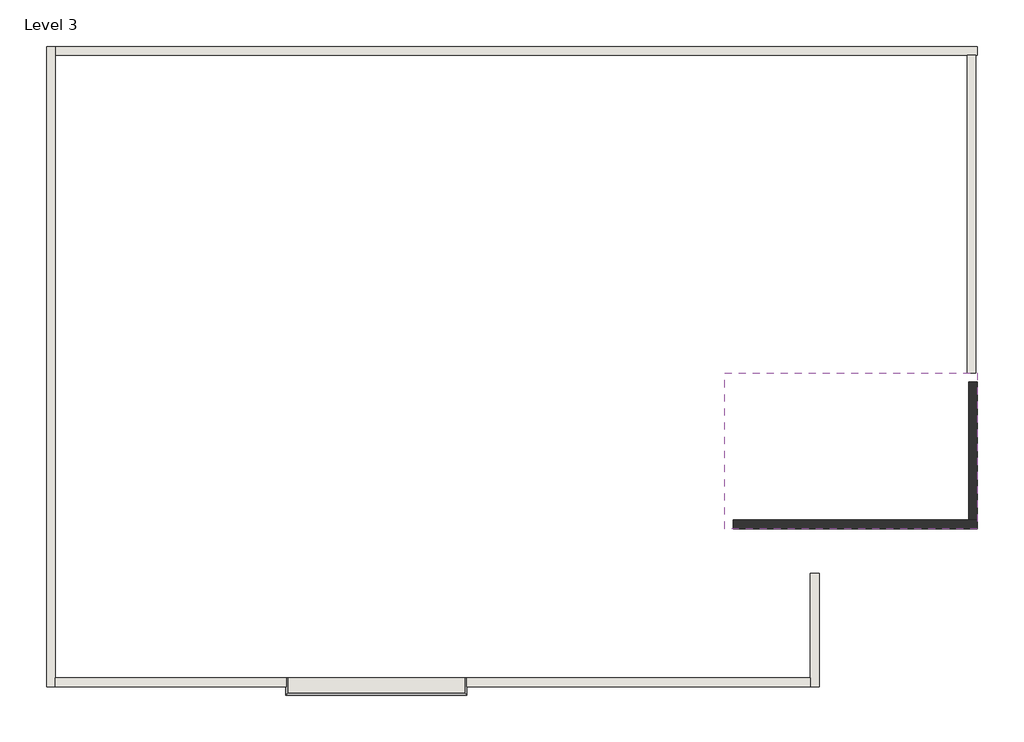
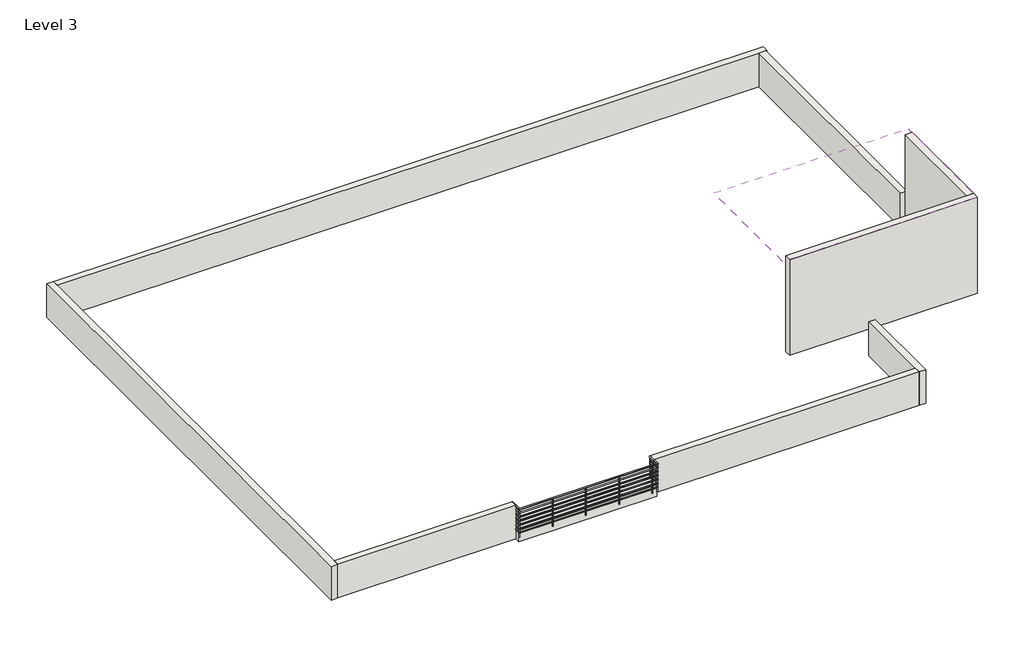
# One storey: 10 walls, 1 covering, 1 railing.
"""IFC4 building model written with IfcOpenShell, lengths in millimetres."""

from ifc_helpers import new_model, si_unit, point, frame, frame_2d, origin, place, context, project, spatial, polyline, circle_curve, ellipse_curve, trimmed, segment, composite_curve, outline, extrude, faceted_brep, transform, mapped, element, save
from ifc_brep_helpers import plane_surface, cylinder_surface, advanced_brep
from components import walls_5_walls_5_63f74a62, walls_6_walls_6_8e6cdcdd

model = new_model("IFC4")

# Units and contexts
model_context = context("Model", 3, world=origin())
ifc_project = project(units=[si_unit("LENGTHUNIT", "METRE", prefix="MILLI")], contexts=[model_context])

# Site, building, storey
site = spatial("IfcSite", under=ifc_project)
building = spatial("IfcBuilding", under=site)
storey = spatial("IfcBuildingStorey", under=building, Name="Level 3", Elevation=3048.0)

# Covering
placement = place(None, origin())
element("IfcCovering", 1, ObjectType="600 x 1200mm grid", at=placement, inside=storey, context=model_context, shape_type="SweptSolid", body=[
    extrude(outline(polyline([(13293.8008502, 3643.3156744), (13293.8008502, 38.1156744), (7439.6639497, 38.1156744), (7439.6639497, 3643.3156744), (13293.8008502, 3643.3156744)])), frame((0.0, 0.0, 6096.0), z_axis=(0.0, 0.0, 1.0), x_axis=(1.0, 0.0, 0.0)), (0.0, 0.0, 1.0), 52.0),
])

# Railing
element("IfcRailing", 2, ObjectType="900mm Pipe", at=placement, inside=storey, context=model_context, shape_type="SolidModel", body=[
    advanced_brep(
    [(-2720.3062226, -3420.8536983, 4095.5083956), (-2680.3062226, -3420.8536983, 4095.5083956), (-2720.3062226, -3815.4929435, 4095.5083956), (-2680.3062226, -3775.4929435, 4095.5083956), (1468.5864069, -3815.4929435, 4095.5083956), (1428.5864069, -3775.4929435, 4095.5083956), (1468.5864069, -3420.8536983, 4095.5083956), (1428.5864069, -3420.8536983, 4095.5083956)],
    [
        (0, 1, circle_curve(frame((-2700.3062226, -3420.8536983, 4095.5083956), z_axis=(0.0, 1.0, 0.0), x_axis=(1.0, 0.0, 0.0)), 20.0)),
        (1, 0, circle_curve(frame((-2700.3062226, -3420.8536983, 4095.5083956), z_axis=(0.0, 1.0, 0.0), x_axis=(1.0, 0.0, 0.0)), 20.0)),
        (0, 2),
        (2, 3, ellipse_curve(frame((-2700.3062226, -3795.4929435, 4095.5083956), z_axis=(-0.7071067811865459, 0.7071067811865491, 0.0), x_axis=(0.7071067811865491, 0.7071067811865458, 0.0)), 28.2842712, 20.0)),
        (3, 1),
        (3, 2, ellipse_curve(frame((-2700.3062226, -3795.4929435, 4095.5083956), z_axis=(-0.7071067811865459, 0.7071067811865491, 0.0), x_axis=(0.7071067811865491, 0.7071067811865458, 0.0)), 28.2842712, 20.0)),
        (2, 4),
        (4, 5, ellipse_curve(frame((1448.5864069, -3795.4929435, 4095.5083956), z_axis=(-0.707106781186549, -0.7071067811865458, 0.0), x_axis=(-0.7071067811865461, 0.7071067811865489, 0.0)), 28.2842712, 20.0)),
        (5, 3),
        (5, 4, ellipse_curve(frame((1448.5864069, -3795.4929435, 4095.5083956), z_axis=(-0.707106781186549, -0.7071067811865458, 0.0), x_axis=(-0.7071067811865461, 0.7071067811865489, 0.0)), 28.2842712, 20.0)),
        (6, 7, circle_curve(frame((1448.5864069, -3420.8536983, 4095.5083956), z_axis=(0.0, 1.0, 0.0), x_axis=(-1.0, 0.0, 0.0)), 20.0)),
        (7, 6, circle_curve(frame((1448.5864069, -3420.8536983, 4095.5083956), z_axis=(0.0, 1.0, 0.0), x_axis=(-1.0, 0.0, 0.0)), 20.0)),
        (4, 6),
        (7, 5),
    ],
    [
        plane_surface(frame((-2700.3062226, -3420.8536983, 4115.5083956), z_axis=(0.0, 1.0, 0.0), x_axis=(0.0, 0.0, -1.0))),
        cylinder_surface(frame((-2700.3062226, -3420.8536983, 4095.5083956), z_axis=(0.0, 1.0, 0.0), x_axis=(1.0, 0.0, 0.0)), 20.0),
        cylinder_surface(frame((-2700.3062226, -3795.4929435, 4095.5083956), z_axis=(-1.0, 0.0, 0.0), x_axis=(0.0, 1.0, 0.0)), 20.0),
        plane_surface(frame((1448.5864069, -3420.8536983, 4115.5083956), z_axis=(0.0, 1.0, 0.0), x_axis=(0.0, 0.0, 1.0))),
        cylinder_surface(frame((1448.5864069, -3795.4929435, 4095.5083956), z_axis=(0.0, -1.0, 0.0), x_axis=(-1.0, 0.0, 0.0)), 20.0),
    ],
    [
        (0, [[1, 2]]),
        (1, [[-1, 3, 4, 5]]),
        (1, [[-2, -5, 6, -3]]),
        (2, [[-4, 7, 8, 9]]),
        (2, [[-6, -9, 10, -7]]),
        (3, [[11, 12]]),
        (4, [[-8, 13, -12, 14]]),
        (4, [[-10, -14, -11, -13]]),
    ],
),
    advanced_brep(
    [(-2685.3062226, -3420.8536983, 3975.5083956), (-2715.3062226, -3420.8536983, 3975.5083956), (-2685.3062226, -3780.4929435, 3975.5083956), (-2715.3062226, -3810.4929435, 3975.5083956), (1433.5864069, -3780.4929435, 3975.5083956), (1463.5864069, -3810.4929435, 3975.5083956), (1433.5864069, -3420.8536983, 3975.5083956), (1463.5864069, -3420.8536983, 3975.5083956)],
    [
        (0, 1, circle_curve(frame((-2700.3062226, -3420.8536983, 3975.5083956), z_axis=(0.0, 1.0, 0.0), x_axis=(-1.0, 0.0, 0.0)), 15.0)),
        (1, 0, circle_curve(frame((-2700.3062226, -3420.8536983, 3975.5083956), z_axis=(0.0, 1.0, 0.0), x_axis=(-1.0, 0.0, 0.0)), 15.0)),
        (0, 2),
        (2, 3, ellipse_curve(frame((-2700.3062226, -3795.4929435, 3975.5083956), z_axis=(-0.7071067811865459, 0.7071067811865491, 0.0), x_axis=(0.7071067811865491, 0.7071067811865458, 0.0)), 21.2132034, 15.0)),
        (3, 1),
        (3, 2, ellipse_curve(frame((-2700.3062226, -3795.4929435, 3975.5083956), z_axis=(-0.7071067811865459, 0.7071067811865491, 0.0), x_axis=(0.7071067811865491, 0.7071067811865458, 0.0)), 21.2132034, 15.0)),
        (2, 4),
        (4, 5, ellipse_curve(frame((1448.5864069, -3795.4929435, 3975.5083956), z_axis=(-0.707106781186549, -0.7071067811865458, 0.0), x_axis=(-0.7071067811865461, 0.7071067811865489, 0.0)), 21.2132034, 15.0)),
        (5, 3),
        (5, 4, ellipse_curve(frame((1448.5864069, -3795.4929435, 3975.5083956), z_axis=(-0.707106781186549, -0.7071067811865458, 0.0), x_axis=(-0.7071067811865461, 0.7071067811865489, 0.0)), 21.2132034, 15.0)),
        (6, 7, circle_curve(frame((1448.5864069, -3420.8536983, 3975.5083956), z_axis=(0.0, 1.0, 0.0), x_axis=(1.0, 0.0, 0.0)), 15.0)),
        (7, 6, circle_curve(frame((1448.5864069, -3420.8536983, 3975.5083956), z_axis=(0.0, 1.0, 0.0), x_axis=(1.0, 0.0, 0.0)), 15.0)),
        (4, 6),
        (7, 5),
    ],
    [
        plane_surface(frame((-2700.3062226, -3420.8536983, 3990.5083956), z_axis=(0.0, 1.0, 0.0), x_axis=(0.0, 0.0, -1.0))),
        cylinder_surface(frame((-2700.3062226, -3420.8536983, 3975.5083956), z_axis=(0.0, 1.0, 0.0), x_axis=(-1.0, 0.0, 0.0)), 15.0),
        cylinder_surface(frame((-2700.3062226, -3795.4929435, 3975.5083956), z_axis=(-1.0, 0.0, 0.0), x_axis=(0.0, -1.0, 0.0)), 15.0),
        plane_surface(frame((1448.5864069, -3420.8536983, 3990.5083956), z_axis=(0.0, 1.0, 0.0), x_axis=(0.0, 0.0, 1.0))),
        cylinder_surface(frame((1448.5864069, -3795.4929435, 3975.5083956), z_axis=(0.0, -1.0, 0.0), x_axis=(1.0, 0.0, 0.0)), 15.0),
    ],
    [
        (0, [[1, 2]]),
        (1, [[-1, 3, 4, 5]]),
        (1, [[-2, -5, 6, -3]]),
        (2, [[-4, 7, 8, 9]]),
        (2, [[-6, -9, 10, -7]]),
        (3, [[11, 12]]),
        (4, [[-8, 13, -12, 14]]),
        (4, [[-10, -14, -11, -13]]),
    ],
),
    advanced_brep(
    [(-2685.3062226, -3420.8536983, 3850.5083956), (-2715.3062226, -3420.8536983, 3850.5083956), (-2685.3062226, -3780.4929435, 3850.5083956), (-2715.3062226, -3810.4929435, 3850.5083956), (1433.5864069, -3780.4929435, 3850.5083956), (1463.5864069, -3810.4929435, 3850.5083956), (1433.5864069, -3420.8536983, 3850.5083956), (1463.5864069, -3420.8536983, 3850.5083956)],
    [
        (0, 1, circle_curve(frame((-2700.3062226, -3420.8536983, 3850.5083956), z_axis=(0.0, 1.0, 0.0), x_axis=(-1.0, 0.0, 0.0)), 15.0)),
        (1, 0, circle_curve(frame((-2700.3062226, -3420.8536983, 3850.5083956), z_axis=(0.0, 1.0, 0.0), x_axis=(-1.0, 0.0, 0.0)), 15.0)),
        (0, 2),
        (2, 3, ellipse_curve(frame((-2700.3062226, -3795.4929435, 3850.5083956), z_axis=(-0.7071067811865459, 0.7071067811865491, 0.0), x_axis=(0.7071067811865491, 0.7071067811865458, 0.0)), 21.2132034, 15.0)),
        (3, 1),
        (3, 2, ellipse_curve(frame((-2700.3062226, -3795.4929435, 3850.5083956), z_axis=(-0.7071067811865459, 0.7071067811865491, 0.0), x_axis=(0.7071067811865491, 0.7071067811865458, 0.0)), 21.2132034, 15.0)),
        (2, 4),
        (4, 5, ellipse_curve(frame((1448.5864069, -3795.4929435, 3850.5083956), z_axis=(-0.707106781186549, -0.7071067811865458, 0.0), x_axis=(-0.7071067811865461, 0.7071067811865489, 0.0)), 21.2132034, 15.0)),
        (5, 3),
        (5, 4, ellipse_curve(frame((1448.5864069, -3795.4929435, 3850.5083956), z_axis=(-0.707106781186549, -0.7071067811865458, 0.0), x_axis=(-0.7071067811865461, 0.7071067811865489, 0.0)), 21.2132034, 15.0)),
        (6, 7, circle_curve(frame((1448.5864069, -3420.8536983, 3850.5083956), z_axis=(0.0, 1.0, 0.0), x_axis=(1.0, 0.0, 0.0)), 15.0)),
        (7, 6, circle_curve(frame((1448.5864069, -3420.8536983, 3850.5083956), z_axis=(0.0, 1.0, 0.0), x_axis=(1.0, 0.0, 0.0)), 15.0)),
        (4, 6),
        (7, 5),
    ],
    [
        plane_surface(frame((-2700.3062226, -3420.8536983, 3865.5083956), z_axis=(0.0, 1.0, 0.0), x_axis=(0.0, 0.0, -1.0))),
        cylinder_surface(frame((-2700.3062226, -3420.8536983, 3850.5083956), z_axis=(0.0, 1.0, 0.0), x_axis=(-1.0, 0.0, 0.0)), 15.0),
        cylinder_surface(frame((-2700.3062226, -3795.4929435, 3850.5083956), z_axis=(-1.0, 0.0, 0.0), x_axis=(0.0, -1.0, 0.0)), 15.0),
        plane_surface(frame((1448.5864069, -3420.8536983, 3865.5083956), z_axis=(0.0, 1.0, 0.0), x_axis=(0.0, 0.0, 1.0))),
        cylinder_surface(frame((1448.5864069, -3795.4929435, 3850.5083956), z_axis=(0.0, -1.0, 0.0), x_axis=(1.0, 0.0, 0.0)), 15.0),
    ],
    [
        (0, [[1, 2]]),
        (1, [[-1, 3, 4, 5]]),
        (1, [[-2, -5, 6, -3]]),
        (2, [[-4, 7, 8, 9]]),
        (2, [[-6, -9, 10, -7]]),
        (3, [[11, 12]]),
        (4, [[-8, 13, -12, 14]]),
        (4, [[-10, -14, -11, -13]]),
    ],
),
    advanced_brep(
    [(-2685.3062226, -3420.8536983, 3725.5083956), (-2715.3062226, -3420.8536983, 3725.5083956), (-2685.3062226, -3780.4929435, 3725.5083956), (-2715.3062226, -3810.4929435, 3725.5083956), (1433.5864069, -3780.4929435, 3725.5083956), (1463.5864069, -3810.4929435, 3725.5083956), (1433.5864069, -3420.8536983, 3725.5083956), (1463.5864069, -3420.8536983, 3725.5083956)],
    [
        (0, 1, circle_curve(frame((-2700.3062226, -3420.8536983, 3725.5083956), z_axis=(0.0, 1.0, 0.0), x_axis=(-1.0, 0.0, 0.0)), 15.0)),
        (1, 0, circle_curve(frame((-2700.3062226, -3420.8536983, 3725.5083956), z_axis=(0.0, 1.0, 0.0), x_axis=(-1.0, 0.0, 0.0)), 15.0)),
        (0, 2),
        (2, 3, ellipse_curve(frame((-2700.3062226, -3795.4929435, 3725.5083956), z_axis=(-0.7071067811865459, 0.7071067811865491, 0.0), x_axis=(0.7071067811865491, 0.7071067811865458, 0.0)), 21.2132034, 15.0)),
        (3, 1),
        (3, 2, ellipse_curve(frame((-2700.3062226, -3795.4929435, 3725.5083956), z_axis=(-0.7071067811865459, 0.7071067811865491, 0.0), x_axis=(0.7071067811865491, 0.7071067811865458, 0.0)), 21.2132034, 15.0)),
        (2, 4),
        (4, 5, ellipse_curve(frame((1448.5864069, -3795.4929435, 3725.5083956), z_axis=(-0.707106781186549, -0.7071067811865458, 0.0), x_axis=(-0.7071067811865461, 0.7071067811865489, 0.0)), 21.2132034, 15.0)),
        (5, 3),
        (5, 4, ellipse_curve(frame((1448.5864069, -3795.4929435, 3725.5083956), z_axis=(-0.707106781186549, -0.7071067811865458, 0.0), x_axis=(-0.7071067811865461, 0.7071067811865489, 0.0)), 21.2132034, 15.0)),
        (6, 7, circle_curve(frame((1448.5864069, -3420.8536983, 3725.5083956), z_axis=(0.0, 1.0, 0.0), x_axis=(1.0, 0.0, 0.0)), 15.0)),
        (7, 6, circle_curve(frame((1448.5864069, -3420.8536983, 3725.5083956), z_axis=(0.0, 1.0, 0.0), x_axis=(1.0, 0.0, 0.0)), 15.0)),
        (4, 6),
        (7, 5),
    ],
    [
        plane_surface(frame((-2700.3062226, -3420.8536983, 3740.5083956), z_axis=(0.0, 1.0, 0.0), x_axis=(0.0, 0.0, -1.0))),
        cylinder_surface(frame((-2700.3062226, -3420.8536983, 3725.5083956), z_axis=(0.0, 1.0, 0.0), x_axis=(-1.0, 0.0, 0.0)), 15.0),
        cylinder_surface(frame((-2700.3062226, -3795.4929435, 3725.5083956), z_axis=(-1.0, 0.0, 0.0), x_axis=(0.0, -1.0, 0.0)), 15.0),
        plane_surface(frame((1448.5864069, -3420.8536983, 3740.5083956), z_axis=(0.0, 1.0, 0.0), x_axis=(0.0, 0.0, 1.0))),
        cylinder_surface(frame((1448.5864069, -3795.4929435, 3725.5083956), z_axis=(0.0, -1.0, 0.0), x_axis=(1.0, 0.0, 0.0)), 15.0),
    ],
    [
        (0, [[1, 2]]),
        (1, [[-1, 3, 4, 5]]),
        (1, [[-2, -5, 6, -3]]),
        (2, [[-4, 7, 8, 9]]),
        (2, [[-6, -9, 10, -7]]),
        (3, [[11, 12]]),
        (4, [[-8, 13, -12, 14]]),
        (4, [[-10, -14, -11, -13]]),
    ],
),
    advanced_brep(
    [(-2685.3062226, -3420.8536983, 3600.5083956), (-2715.3062226, -3420.8536983, 3600.5083956), (-2685.3062226, -3780.4929435, 3600.5083956), (-2715.3062226, -3810.4929435, 3600.5083956), (1433.5864069, -3780.4929435, 3600.5083956), (1463.5864069, -3810.4929435, 3600.5083956), (1433.5864069, -3420.8536983, 3600.5083956), (1463.5864069, -3420.8536983, 3600.5083956)],
    [
        (0, 1, circle_curve(frame((-2700.3062226, -3420.8536983, 3600.5083956), z_axis=(0.0, 1.0, 0.0), x_axis=(-1.0, 0.0, 0.0)), 15.0)),
        (1, 0, circle_curve(frame((-2700.3062226, -3420.8536983, 3600.5083956), z_axis=(0.0, 1.0, 0.0), x_axis=(-1.0, 0.0, 0.0)), 15.0)),
        (0, 2),
        (2, 3, ellipse_curve(frame((-2700.3062226, -3795.4929435, 3600.5083956), z_axis=(-0.7071067811865459, 0.7071067811865491, 0.0), x_axis=(0.7071067811865491, 0.7071067811865458, 0.0)), 21.2132034, 15.0)),
        (3, 1),
        (3, 2, ellipse_curve(frame((-2700.3062226, -3795.4929435, 3600.5083956), z_axis=(-0.7071067811865459, 0.7071067811865491, 0.0), x_axis=(0.7071067811865491, 0.7071067811865458, 0.0)), 21.2132034, 15.0)),
        (2, 4),
        (4, 5, ellipse_curve(frame((1448.5864069, -3795.4929435, 3600.5083956), z_axis=(-0.707106781186549, -0.7071067811865458, 0.0), x_axis=(-0.7071067811865461, 0.7071067811865489, 0.0)), 21.2132034, 15.0)),
        (5, 3),
        (5, 4, ellipse_curve(frame((1448.5864069, -3795.4929435, 3600.5083956), z_axis=(-0.707106781186549, -0.7071067811865458, 0.0), x_axis=(-0.7071067811865461, 0.7071067811865489, 0.0)), 21.2132034, 15.0)),
        (6, 7, circle_curve(frame((1448.5864069, -3420.8536983, 3600.5083956), z_axis=(0.0, 1.0, 0.0), x_axis=(1.0, 0.0, 0.0)), 15.0)),
        (7, 6, circle_curve(frame((1448.5864069, -3420.8536983, 3600.5083956), z_axis=(0.0, 1.0, 0.0), x_axis=(1.0, 0.0, 0.0)), 15.0)),
        (4, 6),
        (7, 5),
    ],
    [
        plane_surface(frame((-2700.3062226, -3420.8536983, 3615.5083956), z_axis=(0.0, 1.0, 0.0), x_axis=(0.0, 0.0, -1.0))),
        cylinder_surface(frame((-2700.3062226, -3420.8536983, 3600.5083956), z_axis=(0.0, 1.0, 0.0), x_axis=(-1.0, 0.0, 0.0)), 15.0),
        cylinder_surface(frame((-2700.3062226, -3795.4929435, 3600.5083956), z_axis=(-1.0, 0.0, 0.0), x_axis=(0.0, -1.0, 0.0)), 15.0),
        plane_surface(frame((1448.5864069, -3420.8536983, 3615.5083956), z_axis=(0.0, 1.0, 0.0), x_axis=(0.0, 0.0, 1.0))),
        cylinder_surface(frame((1448.5864069, -3795.4929435, 3600.5083956), z_axis=(0.0, -1.0, 0.0), x_axis=(1.0, 0.0, 0.0)), 15.0),
    ],
    [
        (0, [[1, 2]]),
        (1, [[-1, 3, 4, 5]]),
        (1, [[-2, -5, 6, -3]]),
        (2, [[-4, 7, 8, 9]]),
        (2, [[-6, -9, 10, -7]]),
        (3, [[11, 12]]),
        (4, [[-8, 13, -12, 14]]),
        (4, [[-10, -14, -11, -13]]),
    ],
),
    advanced_brep(
    [(-2685.3062226, -3420.8536983, 3475.5083956), (-2715.3062226, -3420.8536983, 3475.5083956), (-2685.3062226, -3780.4929435, 3475.5083956), (-2715.3062226, -3810.4929435, 3475.5083956), (1433.5864069, -3780.4929435, 3475.5083956), (1463.5864069, -3810.4929435, 3475.5083956), (1433.5864069, -3420.8536983, 3475.5083956), (1463.5864069, -3420.8536983, 3475.5083956)],
    [
        (0, 1, circle_curve(frame((-2700.3062226, -3420.8536983, 3475.5083956), z_axis=(0.0, 1.0, 0.0), x_axis=(-1.0, 0.0, 0.0)), 15.0)),
        (1, 0, circle_curve(frame((-2700.3062226, -3420.8536983, 3475.5083956), z_axis=(0.0, 1.0, 0.0), x_axis=(-1.0, 0.0, 0.0)), 15.0)),
        (0, 2),
        (2, 3, ellipse_curve(frame((-2700.3062226, -3795.4929435, 3475.5083956), z_axis=(-0.7071067811865459, 0.7071067811865491, 0.0), x_axis=(0.7071067811865491, 0.7071067811865458, 0.0)), 21.2132034, 15.0)),
        (3, 1),
        (3, 2, ellipse_curve(frame((-2700.3062226, -3795.4929435, 3475.5083956), z_axis=(-0.7071067811865459, 0.7071067811865491, 0.0), x_axis=(0.7071067811865491, 0.7071067811865458, 0.0)), 21.2132034, 15.0)),
        (2, 4),
        (4, 5, ellipse_curve(frame((1448.5864069, -3795.4929435, 3475.5083956), z_axis=(-0.707106781186549, -0.7071067811865458, 0.0), x_axis=(-0.7071067811865461, 0.7071067811865489, 0.0)), 21.2132034, 15.0)),
        (5, 3),
        (5, 4, ellipse_curve(frame((1448.5864069, -3795.4929435, 3475.5083956), z_axis=(-0.707106781186549, -0.7071067811865458, 0.0), x_axis=(-0.7071067811865461, 0.7071067811865489, 0.0)), 21.2132034, 15.0)),
        (6, 7, circle_curve(frame((1448.5864069, -3420.8536983, 3475.5083956), z_axis=(0.0, 1.0, 0.0), x_axis=(1.0, 0.0, 0.0)), 15.0)),
        (7, 6, circle_curve(frame((1448.5864069, -3420.8536983, 3475.5083956), z_axis=(0.0, 1.0, 0.0), x_axis=(1.0, 0.0, 0.0)), 15.0)),
        (4, 6),
        (7, 5),
    ],
    [
        plane_surface(frame((-2700.3062226, -3420.8536983, 3490.5083956), z_axis=(0.0, 1.0, 0.0), x_axis=(0.0, 0.0, -1.0))),
        cylinder_surface(frame((-2700.3062226, -3420.8536983, 3475.5083956), z_axis=(0.0, 1.0, 0.0), x_axis=(-1.0, 0.0, 0.0)), 15.0),
        cylinder_surface(frame((-2700.3062226, -3795.4929435, 3475.5083956), z_axis=(-1.0, 0.0, 0.0), x_axis=(0.0, -1.0, 0.0)), 15.0),
        plane_surface(frame((1448.5864069, -3420.8536983, 3490.5083956), z_axis=(0.0, 1.0, 0.0), x_axis=(0.0, 0.0, 1.0))),
        cylinder_surface(frame((1448.5864069, -3795.4929435, 3475.5083956), z_axis=(0.0, -1.0, 0.0), x_axis=(1.0, 0.0, 0.0)), 15.0),
    ],
    [
        (0, [[1, 2]]),
        (1, [[-1, 3, 4, 5]]),
        (1, [[-2, -5, 6, -3]]),
        (2, [[-4, 7, 8, 9]]),
        (2, [[-6, -9, 10, -7]]),
        (3, [[11, 12]]),
        (4, [[-8, 13, -12, 14]]),
        (4, [[-10, -14, -11, -13]]),
    ],
),
    advanced_brep(
    [(-2685.3062226, -3420.8536983, 3350.5083956), (-2715.3062226, -3420.8536983, 3350.5083956), (-2685.3062226, -3780.4929435, 3350.5083956), (-2715.3062226, -3810.4929435, 3350.5083956), (1433.5864069, -3780.4929435, 3350.5083956), (1463.5864069, -3810.4929435, 3350.5083956), (1433.5864069, -3420.8536983, 3350.5083956), (1463.5864069, -3420.8536983, 3350.5083956)],
    [
        (0, 1, circle_curve(frame((-2700.3062226, -3420.8536983, 3350.5083956), z_axis=(0.0, 1.0, 0.0), x_axis=(-1.0, 0.0, 0.0)), 15.0)),
        (1, 0, circle_curve(frame((-2700.3062226, -3420.8536983, 3350.5083956), z_axis=(0.0, 1.0, 0.0), x_axis=(-1.0, 0.0, 0.0)), 15.0)),
        (0, 2),
        (2, 3, ellipse_curve(frame((-2700.3062226, -3795.4929435, 3350.5083956), z_axis=(-0.7071067811865459, 0.7071067811865491, 0.0), x_axis=(0.7071067811865491, 0.7071067811865458, 0.0)), 21.2132034, 15.0)),
        (3, 1),
        (3, 2, ellipse_curve(frame((-2700.3062226, -3795.4929435, 3350.5083956), z_axis=(-0.7071067811865459, 0.7071067811865491, 0.0), x_axis=(0.7071067811865491, 0.7071067811865458, 0.0)), 21.2132034, 15.0)),
        (2, 4),
        (4, 5, ellipse_curve(frame((1448.5864069, -3795.4929435, 3350.5083956), z_axis=(-0.707106781186549, -0.7071067811865458, 0.0), x_axis=(-0.7071067811865461, 0.7071067811865489, 0.0)), 21.2132034, 15.0)),
        (5, 3),
        (5, 4, ellipse_curve(frame((1448.5864069, -3795.4929435, 3350.5083956), z_axis=(-0.707106781186549, -0.7071067811865458, 0.0), x_axis=(-0.7071067811865461, 0.7071067811865489, 0.0)), 21.2132034, 15.0)),
        (6, 7, circle_curve(frame((1448.5864069, -3420.8536983, 3350.5083956), z_axis=(0.0, 1.0, 0.0), x_axis=(1.0, 0.0, 0.0)), 15.0)),
        (7, 6, circle_curve(frame((1448.5864069, -3420.8536983, 3350.5083956), z_axis=(0.0, 1.0, 0.0), x_axis=(1.0, 0.0, 0.0)), 15.0)),
        (4, 6),
        (7, 5),
    ],
    [
        plane_surface(frame((-2700.3062226, -3420.8536983, 3365.5083956), z_axis=(0.0, 1.0, 0.0), x_axis=(0.0, 0.0, -1.0))),
        cylinder_surface(frame((-2700.3062226, -3420.8536983, 3350.5083956), z_axis=(0.0, 1.0, 0.0), x_axis=(-1.0, 0.0, 0.0)), 15.0),
        cylinder_surface(frame((-2700.3062226, -3795.4929435, 3350.5083956), z_axis=(-1.0, 0.0, 0.0), x_axis=(0.0, -1.0, 0.0)), 15.0),
        plane_surface(frame((1448.5864069, -3420.8536983, 3365.5083956), z_axis=(0.0, 1.0, 0.0), x_axis=(0.0, 0.0, 1.0))),
        cylinder_surface(frame((1448.5864069, -3795.4929435, 3350.5083956), z_axis=(0.0, -1.0, 0.0), x_axis=(1.0, 0.0, 0.0)), 15.0),
    ],
    [
        (0, [[1, 2]]),
        (1, [[-1, 3, 4, 5]]),
        (1, [[-2, -5, 6, -3]]),
        (2, [[-4, 7, 8, 9]]),
        (2, [[-6, -9, 10, -7]]),
        (3, [[11, 12]]),
        (4, [[-8, 13, -12, 14]]),
        (4, [[-10, -14, -11, -13]]),
    ],
),
    extrude(outline(composite_curve([segment(trimmed(circle_curve(frame_2d((1299.6937774, -3795.4929435)), 12.5), [point((1299.6937774, -3782.9929435))], [point((1299.6937774, -3807.9929435))], False, "CARTESIAN"), True, "CONTINUOUS"), segment(trimmed(circle_curve(frame_2d((1299.6937774, -3795.4929435)), 12.5), [point((1299.6937774, -3807.9929435))], [point((1299.6937774, -3782.9929435))], False, "CARTESIAN"), True, "CONTINUOUS")], self_intersect=False)), frame((0.0, 0.0, 3215.5083956), z_axis=(0.0, 0.0, 1.0), x_axis=(1.0, 0.0, 0.0)), (0.0, 0.0, 1.0), 860.0),
    extrude(outline(composite_curve([segment(trimmed(circle_curve(frame_2d((299.6937774, -3795.4929435)), 12.5), [point((299.6937774, -3782.9929435))], [point((299.6937774, -3807.9929435))], False, "CARTESIAN"), True, "CONTINUOUS"), segment(trimmed(circle_curve(frame_2d((299.6937774, -3795.4929435)), 12.5), [point((299.6937774, -3807.9929435))], [point((299.6937774, -3782.9929435))], False, "CARTESIAN"), True, "CONTINUOUS")], self_intersect=False)), frame((0.0, 0.0, 3215.5083956), z_axis=(0.0, 0.0, 1.0), x_axis=(1.0, 0.0, 0.0)), (0.0, 0.0, 1.0), 860.0),
    extrude(outline(composite_curve([segment(trimmed(circle_curve(frame_2d((-700.3062226, -3795.4929435)), 12.5), [point((-700.3062226, -3782.9929435))], [point((-700.3062226, -3807.9929435))], False, "CARTESIAN"), True, "CONTINUOUS"), segment(trimmed(circle_curve(frame_2d((-700.3062226, -3795.4929435)), 12.5), [point((-700.3062226, -3807.9929435))], [point((-700.3062226, -3782.9929435))], False, "CARTESIAN"), True, "CONTINUOUS")], self_intersect=False)), frame((0.0, 0.0, 3215.5083956), z_axis=(0.0, 0.0, 1.0), x_axis=(1.0, 0.0, 0.0)), (0.0, 0.0, 1.0), 860.0),
    extrude(outline(composite_curve([segment(trimmed(circle_curve(frame_2d((-1700.3062226, -3795.4929435)), 12.5), [point((-1700.3062226, -3782.9929435))], [point((-1700.3062226, -3807.9929435))], False, "CARTESIAN"), True, "CONTINUOUS"), segment(trimmed(circle_curve(frame_2d((-1700.3062226, -3795.4929435)), 12.5), [point((-1700.3062226, -3807.9929435))], [point((-1700.3062226, -3782.9929435))], False, "CARTESIAN"), True, "CONTINUOUS")], self_intersect=False)), frame((0.0, 0.0, 3215.5083956), z_axis=(0.0, 0.0, 1.0), x_axis=(1.0, 0.0, 0.0)), (0.0, 0.0, 1.0), 860.0),
    extrude(outline(composite_curve([segment(trimmed(circle_curve(frame_2d((1448.5864069, -3795.4929435)), 12.5), [point((1448.5864069, -3782.9929435))], [point((1448.5864069, -3807.9929435))], False, "CARTESIAN"), True, "CONTINUOUS"), segment(trimmed(circle_curve(frame_2d((1448.5864069, -3795.4929435)), 12.5), [point((1448.5864069, -3807.9929435))], [point((1448.5864069, -3782.9929435))], False, "CARTESIAN"), True, "CONTINUOUS")], self_intersect=False)), frame((0.0, 0.0, 3215.5083956), z_axis=(0.0, 0.0, 1.0), x_axis=(1.0, 0.0, 0.0)), (0.0, 0.0, 1.0), 860.0),
    extrude(outline(composite_curve([segment(trimmed(circle_curve(frame_2d((-2700.3062226, -3795.4929435)), 12.5), [point((-2687.8062226, -3795.4929435))], [point((-2712.8062226, -3795.4929435))], False, "CARTESIAN"), True, "CONTINUOUS"), segment(trimmed(circle_curve(frame_2d((-2700.3062226, -3795.4929435)), 12.5), [point((-2712.8062226, -3795.4929435))], [point((-2687.8062226, -3795.4929435))], False, "CARTESIAN"), True, "CONTINUOUS")], self_intersect=False)), frame((0.0, 0.0, 3215.5083956), z_axis=(0.0, 0.0, 1.0), x_axis=(1.0, 0.0, 0.0)), (0.0, 0.0, 1.0), 860.0),
    extrude(outline(composite_curve([segment(trimmed(circle_curve(frame_2d((1448.5864069, -3433.3536983)), 12.5), [point((1436.0864069, -3433.3536983))], [point((1461.0864069, -3433.3536983))], False, "CARTESIAN"), True, "CONTINUOUS"), segment(trimmed(circle_curve(frame_2d((1448.5864069, -3433.3536983)), 12.5), [point((1461.0864069, -3433.3536983))], [point((1436.0864069, -3433.3536983))], False, "CARTESIAN"), True, "CONTINUOUS")], self_intersect=False)), frame((0.0, 0.0, 3215.5083956), z_axis=(0.0, 0.0, 1.0), x_axis=(1.0, 0.0, 0.0)), (0.0, 0.0, 1.0), 860.0),
    extrude(outline(composite_curve([segment(trimmed(circle_curve(frame_2d((-2700.3062226, -3433.3536983)), 12.5), [point((-2687.8062226, -3433.3536983))], [point((-2712.8062226, -3433.3536983))], False, "CARTESIAN"), True, "CONTINUOUS"), segment(trimmed(circle_curve(frame_2d((-2700.3062226, -3433.3536983)), 12.5), [point((-2712.8062226, -3433.3536983))], [point((-2687.8062226, -3433.3536983))], False, "CARTESIAN"), True, "CONTINUOUS")], self_intersect=False)), frame((0.0, 0.0, 3215.5083956), z_axis=(0.0, 0.0, 1.0), x_axis=(1.0, 0.0, 0.0)), (0.0, 0.0, 1.0), 860.0),
])

# Walls
element("IfcWall", 3, ObjectType="Generic - 9\"", at=placement, inside=storey, context=model_context, shape_type="Brep", body=[
    faceted_brep([(7639.6639497, 38.1156744, 3048.0), (13293.8008502, 38.1156744, 3048.0), (13293.8008502, 38.1156744, 6096.0), (7639.6639497, 38.1156744, 6096.0), (7639.6639497, 238.1156744, 3048.0), (7639.6639497, 238.1156744, 6096.0), (13093.8008502, 238.1156744, 6096.0), (13293.8008502, 238.1156744, 6096.0), (13293.8008502, 238.1156744, 3048.0), (13093.8008502, 238.1156744, 3048.0)], [[[0, 1, 2, 3]], [[4, 5, 6, 7, 8, 9]], [[1, 0, 4, 9, 8]], [[3, 2, 7, 6, 5]], [[0, 3, 5, 4]], [[2, 1, 8, 7]]]),
])
element("IfcWall", 4, ObjectType="Generic - 9\"", at=placement, inside=storey, context=model_context, shape_type="Brep", body=[
    faceted_brep([(-8260.4509113, 11210.9156744, 3048.0), (-8260.4509113, -3620.8536983, 3048.0), (-8260.4509113, -3620.8536983, 4114.8), (-8260.4509113, 11210.9156744, 4114.8), (-8060.4509113, 11210.9156744, 3048.0), (-8060.4509113, 11210.9156744, 4114.8), (-8060.4509113, 11010.9156744, 4114.8), (-8060.4509113, -3420.8536983, 4114.8), (-8060.4509113, -3620.8536983, 4114.8), (-8060.4509113, -3620.8536983, 3048.0), (-8060.4509113, -3420.8536983, 3048.0), (-8060.4509113, 11010.9156744, 3048.0)], [[[0, 1, 2, 3]], [[4, 5, 6, 7, 8, 9, 10, 11]], [[1, 0, 4, 11, 10, 9]], [[3, 2, 8, 7, 6, 5]], [[0, 3, 5, 4]], [[2, 1, 9, 8]]]),
])
element("IfcWall", 5, ObjectType="Generic - 9\"", at=placement, inside=storey, context=model_context, shape_type="Brep", body=[
    faceted_brep([(-8060.4509113, 11010.9156744, 3048.0), (13053.0639497, 11010.9156744, 3048.0), (13253.0639497, 11010.9156744, 3048.0), (13293.8008502, 11010.9156744, 3048.0), (13293.8008502, 11010.9156744, 4114.8), (13253.0639497, 11010.9156744, 4114.8), (13053.0639497, 11010.9156744, 4114.8), (-8060.4509113, 11010.9156744, 4114.8), (-8060.4509113, 11210.9156744, 3048.0), (-8060.4509113, 11210.9156744, 4114.8), (13293.8008502, 11210.9156744, 4114.8), (13293.8008502, 11210.9156744, 3048.0)], [[[0, 1, 2, 3, 4, 5, 6, 7]], [[8, 9, 10, 11]], [[3, 2, 1, 0, 8, 11]], [[4, 3, 11, 10]], [[7, 6, 5, 4, 10, 9]], [[0, 7, 9, 8]]]),
])
element("IfcWall", 6, ObjectType="Generic - 9\"", at=placement, inside=storey, context=model_context, shape_type="SweptSolid", body=[
    extrude(outline(polyline([(13053.0639497, 3643.3156744), (13053.0639497, 11010.9156744), (13253.0639497, 11010.9156744), (13253.0639497, 3643.3156744), (13053.0639497, 3643.3156744)])), frame((0.0, 0.0, 3048.0), z_axis=(0.0, 0.0, 1.0), x_axis=(1.0, 0.0, 0.0)), (0.0, 0.0, 1.0), 1066.8),
])
element("IfcWall", 7, ObjectType="Generic - 9\"", at=placement, inside=storey, context=model_context, shape_type="Brep", body=[
    faceted_brep([(9425.7864069, -1001.5101069, 3048.0), (9425.7864069, -3420.8536983, 3048.0), (9425.7864069, -3620.8536983, 3048.0), (9425.7864069, -3620.8536983, 4114.8), (9425.7864069, -3420.8536983, 4114.8), (9425.7864069, -1001.5101069, 4114.8), (9625.7864069, -1001.5101069, 3048.0), (9625.7864069, -1001.5101069, 4114.8), (9625.7864069, -3620.8536983, 4114.8), (9625.7864069, -3620.8536983, 3048.0)], [[[0, 1, 2, 3, 4, 5]], [[6, 7, 8, 9]], [[2, 1, 0, 6, 9]], [[5, 4, 3, 8, 7]], [[0, 5, 7, 6]], [[3, 2, 9, 8]]]),
])
element("IfcWall", 8, ObjectType="Generic - 9\"", at=placement, inside=storey, context=model_context, shape_type="SweptSolid", body=[
    extrude(outline(polyline([(-2702.0878119, -3620.8536983), (-8060.4509113, -3620.8536983), (-8060.4509113, -3420.8536983), (-2702.0878119, -3420.8536983), (-2702.0878119, -3620.8536983)])), frame((0.0, 0.0, 3048.0), z_axis=(0.0, 0.0, 1.0), x_axis=(1.0, 0.0, 0.0)), (0.0, 0.0, 1.0), 1066.8),
])
element("IfcWall", 9, ObjectType="Generic - 9\"", at=placement, inside=storey, context=model_context, shape_type="SweptSolid", body=[
    extrude(outline(polyline([(1448.5864069, -3420.8536983), (9425.7864069, -3420.8536983), (9425.7864069, -3620.8536983), (1448.5864069, -3620.8536983), (1448.5864069, -3420.8536983)])), frame((0.0, 0.0, 3048.0), z_axis=(0.0, 0.0, 1.0), x_axis=(1.0, 0.0, 0.0)), (0.0, 0.0, 1.0), 1066.8),
])
element("IfcWall", 10, ObjectType="Generic - 9\"", at=placement, inside=storey, context=model_context, shape_type="Brep", body=[
    faceted_brep([(13093.8008502, 3443.3156744, 3048.0), (13093.8008502, 238.1156744, 3048.0), (13093.8008502, 238.1156744, 6096.0), (13093.8008502, 3443.3156744, 6096.0), (13293.8008502, 3443.3156744, 3048.0), (13293.8008502, 3443.3156744, 6096.0), (13293.8008502, 238.1156744, 6096.0), (13293.8008502, 238.1156744, 3048.0), (13253.0639497, 3443.3156744, 3048.0)], [[[0, 1, 2, 3]], [[4, 5, 6, 7]], [[1, 0, 8, 4, 7]], [[3, 2, 6, 5]], [[2, 1, 7, 6]], [[0, 3, 5, 4, 8]]]),
])
walls_5_walls_5_shape = walls_5_walls_5_63f74a62(model_context)
element("IfcWall", 11, ObjectType="Walls 5 : Walls 5", at=placement, inside=storey, context=model_context, shape_type="MappedRepresentation", body=[
    mapped(walls_5_walls_5_shape, transform((0.0, 0.0, 0.0), x_axis=(1.0, 0.0, 0.0), y_axis=(0.0, 1.0, 0.0), z_axis=(0.0, 0.0, 1.0))),
])
walls_6_walls_6_shape = walls_6_walls_6_8e6cdcdd(model_context)
element("IfcWall", 12, ObjectType="Walls 6 : Walls 6", at=placement, inside=storey, context=model_context, shape_type="MappedRepresentation", body=[
    mapped(walls_6_walls_6_shape, transform((0.0, 0.0, 0.0), x_axis=(1.0, 0.0, 0.0), y_axis=(0.0, 1.0, 0.0), z_axis=(0.0, 0.0, 1.0))),
])

save(model, "model.ifc")

# Revit data of these elements
# Type "600 x 1200mm grid"
#   built-in parameter 1002203 = 1 (stored number, unit not read)
#   built-in parameter 1002202 = 1 (stored number, unit not read)
#   Layers, outside or top first: 0' - 1.41732" "Default" (function 1); 0' - 0.62992" "Ceiling Tile 600 x 1200" (function 5)
# Type "900mm Pipe"
#   built-in parameter 1008612 = 0.019685 (stored number, unit not read)
#   built-in parameter 1008611 = 0.0984252 (stored number, unit not read)
#   built-in parameter 1008609 = 6.56168 (stored number, unit not read)
#   built-in parameter 1008604 = 0.19685 (stored number, unit not read)
#   built-in parameter 1008603 = 0.164042 (stored number, unit not read)
#   Railing Height = 2' - 11.43307"
#   built-in parameter 1008630 = 2
#   built-in parameter 1008610 = 2
#   built-in parameter 1008605 = 1
#   built-in parameter 1008618 = M_Baluster - Round : 25mm
# Type "Generic - 9\""
#   Layers, outside or top first: 0' - 7.87402" no material (function 1)
# Element 1 (IfcCovering, "600 x 1200mm grid")
#   Height Offset From Level = 10' - 0"
#   Phase Created = New Construction
#   Materials on its faces: "Ceiling Tile 600 x 1200", "Default"
# Element 2 (IfcRailing, "900mm Pipe")
#   built-in parameter 1008621 = 0.549568 (stored number, unit not read)
#   Phase Created = New Construction
# Elements 3, 10 (IfcWall, "Generic - 9\"")
#   Top Offset = 0' - 0"
#   Base Offset = 0' - 0"
#   Unconnected Height = 10' - 0"
#   wall height = 10' - 0"
#   Phase Created = New Construction
#   Base Constraint = Level 3
#   Materials on its faces: "Default Wall"
# Elements 4, 5, 6, 7, 8, 9 (IfcWall, "Generic - 9\"")
#   Top Offset = 0' - 0"
#   Base Offset = 0' - 0"
#   Unconnected Height = 3' - 6"
#   wall height = 3' - 6"
#   Phase Created = New Construction
#   Base Constraint = Level 3
#   Materials on its faces: "Default Wall"
# Element 11 (IfcWall, "Walls 5 : Walls 5")
#   Phase Created = New Construction
#   Materials on its faces: "Default Wall"
# Element 12 (IfcWall, "Walls 6 : Walls 6")
#   Phase Created = New Construction
#   Materials on its faces: "Default Wall"
# Materials
#   "Default": colour RGB 80 80 80, transparency 0
#   "Ceiling Tile 600 x 1200": class "Generic", colour RGB 179 178 175, transparency 0, Description = "Acoustic ceiling tile", Cost = 0
#   "Default Wall": colour RGB 80 80 80, transparency 0
